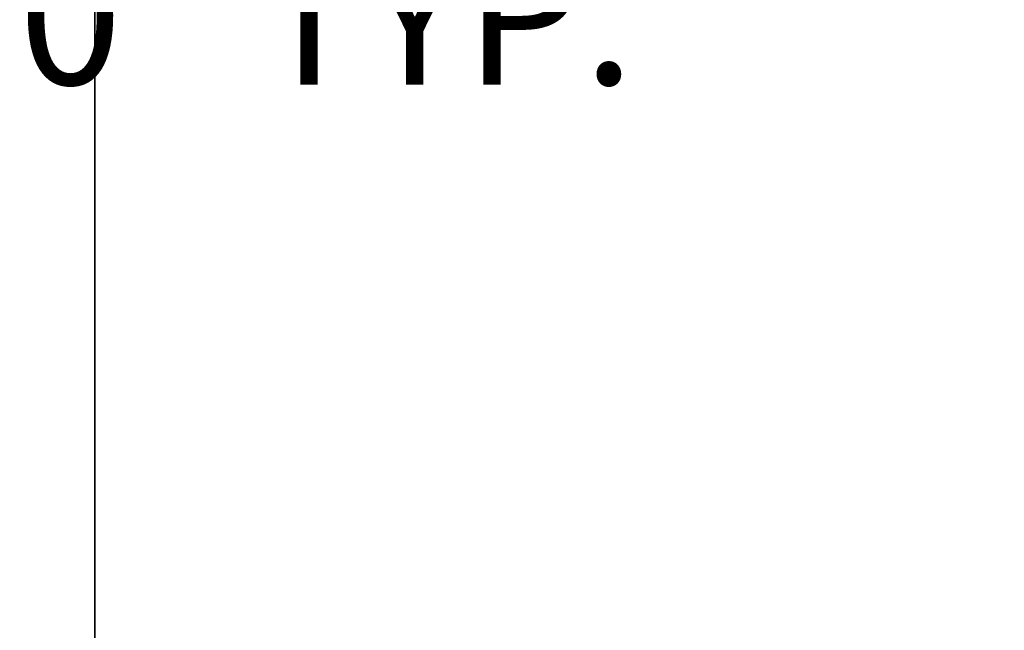
# Model space of a CAD drawing. Units: inches. Extents: x 844 to 2234, y 346 to 1084.
# Tile 4 of 93: x 1093 to 1136, y 627 to 653. Entities that reach past the tile are written whole.
import ezdxf

# ---------------------------------------------------------------- set-up
doc = ezdxf.new("R2010")
doc.units = ezdxf.units.IN
doc.header["$MEASUREMENT"] = 0
doc.layers.add('A-ANNO-DIMS', color=2, linetype='Continuous', lineweight=18)
doc.layers.add('A-WALL', color=7, linetype='Continuous', lineweight=35)
doc.styles.get("Standard").update_dxf_attribs({"font": 'arial.ttf'})
doc.dimstyles.get("Standard").update_dxf_attribs({"dimtxt": 6, "dimasz": 3, "dimexe": 0.18, "dimexo": 0.0625, "dimgap": 0.09, "dimtad": 0, "dimtih": 1, "dimtoh": 1, "dimdec": 1, "dimzin": 0, "dimdsep": 46, "dimlunit": 3, "dimtxsty": 'Standard', "dimblk": 'ARCHTICK', "dimcen": 0.09, "dimadec": 0, "dimazin": 0, "dimtfac": 1, "dimtdec": 1, "dimtofl": 0, "dimtmove": 0, "dimatfit": 3, "dimfxl": 1, "dimtolj": 1, "dimtzin": 0, "dimarcsym": 0})

# ---------------------------------------------------------------- blocks, each defined once
blk = doc.blocks.new('_ArchTick')
at = {"color": 0, "linetype": 'ByBlock', "const_width": 0.15}
blk.add_lwpolyline([(-0.5, -0.5), (0.5, 0.5)], dxfattribs=at)
blk = doc.blocks.new('*D107')
at = {"layer": 'A-ANNO-DIMS', "color": 0, "lineweight": -2, "transparency": 16777216}
for p, q in [((983.442, 646.516), (983.442, 653.834)), ((1031.442, 646.516), (1031.442, 653.834)), ((983.442, 653.654), (1031.442, 653.654)), ((1031.442, 653.654), (1034.442, 653.654))]:
    blk.add_line(p, q, dxfattribs=at)
at = {"layer": 'Defpoints', "color": 0, "transparency": 16777216}
for p in [(1031.442, 653.654), (983.442, 646.454), (1031.442, 646.454)]:
    blk.add_point(p, dxfattribs=at)
at = {"layer": 'A-ANNO-DIMS', "color": 0, "lineweight": -2, "transparency": 16777216, "xscale": 3, "yscale": 3, "zscale": 3, "rotation": 180}
blk.add_blockref('_ArchTick', (983.442, 653.654), dxfattribs=at)
at = {"layer": 'A-ANNO-DIMS', "color": 0, "lineweight": -2, "transparency": 16777216, "xscale": 3, "yscale": 3, "zscale": 3}
blk.add_blockref('_ArchTick', (1031.442, 653.654), dxfattribs=at)
at = {"layer": 'A-ANNO-DIMS', "color": 0, "transparency": 16777216, "insert": (1078.787, 653.654), "char_height": 6, "attachment_point": 5}
blk.add_mtext('\\A1;WARDROBE 4\'-0" TYP.', dxfattribs=at)
blk = doc.blocks.new('*D144')
at = {"layer": 'A-ANNO-DIMS', "color": 0, "lineweight": -2, "transparency": 16777216}
for p, q in [((1096.616, 439.373), (1096.616, 1074.743)), ((1143.116, 492.373), (1143.116, 1074.743)), ((1096.616, 1074.563), (1102.482, 1074.563)), ((1143.116, 1074.563), (1137.25, 1074.563))]:
    blk.add_line(p, q, dxfattribs=at)
at = {"layer": 'Defpoints', "color": 0, "transparency": 16777216}
for p in [(1143.116, 1074.563), (1143.116, 492.311), (1096.616, 439.311)]:
    blk.add_point(p, dxfattribs=at)
at = {"layer": 'A-ANNO-DIMS', "color": 0, "lineweight": -2, "transparency": 16777216, "xscale": 3, "yscale": 3, "zscale": 3, "rotation": 180}
blk.add_blockref('_ArchTick', (1096.616, 1074.563), dxfattribs=at)
at = {"layer": 'A-ANNO-DIMS', "color": 0, "lineweight": -2, "transparency": 16777216, "xscale": 3, "yscale": 3, "zscale": 3}
blk.add_blockref('_ArchTick', (1143.116, 1074.563), dxfattribs=at)
at = {"layer": 'A-ANNO-DIMS', "color": 0, "transparency": 16777216, "insert": (1119.866, 1074.563), "char_height": 6, "attachment_point": 5}
blk.add_mtext('\\A1;3\'-10 1/2"', dxfattribs=at)

msp = doc.modelspace()

# ---------------------------------------------------------------- linework, layer by layer
at = {"layer": 'A-WALL'}
msp.add_line((1096.616, 761.311), (1096.616, 624.311), dxfattribs=at)

# ---------------------------------------------------------------- dimensions: what is measured, and where the dimension line sits
at = {"layer": 'A-ANNO-DIMS'}
dim = msp.add_linear_dim(base=(1143.116, 1074.563), p1=(1096.616, 439.311), p2=(1143.116, 492.311), dimstyle='Standard', override={"dimdec": 1, "dimlfac": 1, "dimrnd": 0, "dimzin": 1, "dimdsep": 46, "dimlunit": 4, "dimfrac": 2}, dxfattribs=at)
dim.commit()
dim.dimension.update_dxf_attribs({"geometry": '*D144', "text_midpoint": (1119.866, 1074.563)})
dim = msp.add_linear_dim(base=(1031.442, 653.654), p1=(983.442, 646.454), p2=(1031.442, 646.454), text='WARDROBE <> TYP.', dimstyle='Standard', override={"dimdec": 1, "dimlfac": 1, "dimrnd": 0, "dimzin": 1, "dimdsep": 46, "dimlunit": 4, "dimfrac": 2}, dxfattribs=at)
dim.commit()
dim.dimension.update_dxf_attribs({"geometry": '*D107', "text_midpoint": (1078.787, 653.654)})

doc.saveas('drawing.dxf')
